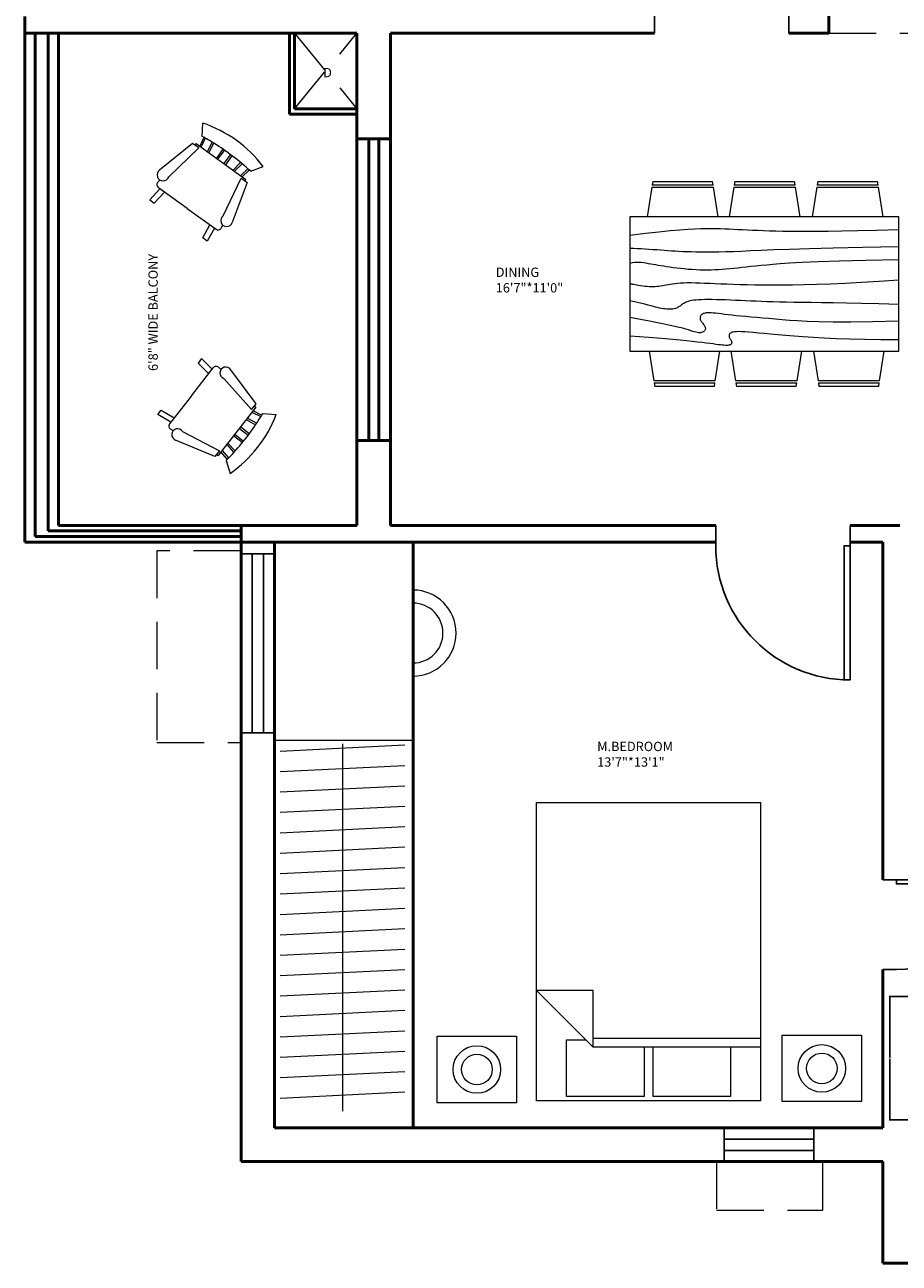
# Model space of a CAD drawing. Units: inches. Extents: x 4795 to 6024, y 2716 to 5025.
# Tile 9 of 19: x 4835 to 5069, y 3894 to 4226. Entities that reach past the tile are written whole.
import ezdxf

# ---------------------------------------------------------------- set-up
doc = ezdxf.new("R2010")
doc.units = ezdxf.units.IN
doc.linetypes.add('DASHED', pattern=[19.05, 12.7, -6.35])
for name, color, linetype, lineweight in [('A-ANNO-DIMS', 2, 'Continuous', 18), ('A-ANNO-TEXT', 7, 'Continuous', 18), ('A-AREA-IDEN', 3, 'Continuous', 18), ('A-DOOR', 4, 'Continuous', 25), ('A-FURN', 8, 'Continuous', 18), ('A-GLAZ', 4, 'Continuous', 25), ('A-WALL', 7, 'Continuous', 50), ('A-WALL-OVHD', 8, 'DASHED', 18)]:
    doc.layers.add(name, color=color, linetype=linetype, lineweight=lineweight)
doc.styles.get("Standard").update_dxf_attribs({"font": 'arial.ttf'})
doc.dimstyles.get("Standard").update_dxf_attribs({"dimtxt": 0.18, "dimasz": 0.18, "dimexe": 0.18, "dimexo": 0.0625, "dimgap": 0.09, "dimtad": 0, "dimtih": 1, "dimtoh": 1, "dimdec": 4, "dimzin": 0, "dimdsep": 46, "dimtxsty": 'Standard', "dimcen": 0.09, "dimadec": 0, "dimazin": 0, "dimtfac": 1, "dimtdec": 4, "dimtofl": 0, "dimtmove": 0, "dimatfit": 3, "dimfxl": 1, "dimtolj": 1, "dimtzin": 0, "dimarcsym": 0})

# ---------------------------------------------------------------- blocks, each defined once
blk = doc.blocks.new('*U2')
for p, q in [((0, 0), (0, -6)), ((40, 0), (40, -6))]:
    blk.add_line(p, q)
blk.add_lwpolyline([(0, 0), (0, 40), (1.75, 40), (1.75, 0)], close=True)
blk.add_arc((0, 0), 40, 0, 90)
blk = doc.blocks.new('Bed - Queen')
for p, q in [((0, -80.00003), (0, 0)), ((0, 0), (59.99999, 0)), ((59.99999, 0), (59.99999, -80.00003)), ((7.99999, -1.2), (28.79998, -1.2)), ((7.99999, -14.4), (7.99999, -1.2)), ((28.79998, -1.2), (28.79998, -14.4)), ((31.19999, -1.2), (51.99999, -1.2)), ((31.19999, -14.4), (31.19999, -1.2)), ((51.99999, -1.2), (51.99999, -16.4)), ((0, -14.4), (44.8, -14.4)), ((59.99999, -29.6), (44.8, -14.4)), ((44.8, -14.4), (44.8, -29.6)), ((51.99999, -16.4), (46.79936, -16.4)), ((44.8, -16.8), (0, -16.8)), ((44.8, -29.6), (59.99999, -29.6)), ((59.99999, -80.00003), (0, -80.00003))]:
    blk.add_line(p, q)
blk = doc.blocks.new('Chair - Rocking')
for p, q in [((-8, -4.5), (-10, -1.5)), ((8, -4.5), (10, -1.5)), ((-7.5, -4.5), (-7, -7)), ((-6.5, -7), (-7.02225, -4.43)), ((-4.5, -7), (-4.96674, -4.19951)), ((-4, -7), (-4.40532, -4.16272)), ((-1.5, -4.05012), (-1.5, -7)), ((-1, -7), (-1, -4.05012)), ((1, -7), (1, -4.04655)), ((1.5, -4.05012), (1.5, -7)), ((4, -7), (4.40187, -4.18694)), ((4.5, -7), (4.96761, -4.19437)), ((6.5, -7), (7, -4.4057)), ((7.5, -4.5), (7, -7)), ((-9, -7.5), (-12, -18.49999)), ((-7, -7.5), (-9, -7.5)), ((-9, -18.49999), (-7, -7.5)), ((-8.23428, -6.99939), (-8.3093, -7.47958)), ((-8.23041, -7), (8.23915, -7)), ((7, -7.5), (9, -7.5)), ((9, -18.49999), (7, -7.5)), ((8.31071, -7.48854), (8.23449, -7.00073)), ((9, -7.5), (12, -18.49999)), ((-10.36644, -20.64523), (-10.5, -21.49999)), ((-9, -22.49999), (-9.5, -26.49999)), ((0, -22.49999), (-9.5, -22.49999)), ((-8, -26.49999), (-7.5, -22.49999)), ((0, -22.49999), (9.5, -22.49999)), ((8, -26.49999), (7.5, -22.49999)), ((9, -22.49999), (9.5, -26.49999)), ((10.5, -21.49999), (10.3575, -20.58798)), ((-9.5, -26.49999), (-8, -26.49999)), ((9.5, -26.49999), (8, -26.49999))]:
    blk.add_line(p, q)
for centre, radius, start, end in [((0, -34.08333), 34.08333, 72.93847, 107.0615), ((0, -68.25004), 64.25, 93.92211, 97.15267), ((0, -68.25004), 64.25, 82.84733, 93.92211), ((-10.5, -18.99999), 1.58114, 161.5651, 18.43495), ((10.5, -18.99999), 1.58114, 161.5651, 18.43495), ((-9.5, -21.49999), 1, 180, 270), ((9.5, -21.49999), 1, 270, 0)]:
    blk.add_arc(centre, radius, start, end)
blk = doc.blocks.new('WIN-48')
for p, q in [((0, 0), (0, 48)), ((0, 48), (9, 48)), ((3, 0), (3, 48)), ((6, 48), (6, 0)), ((9, 48), (9, 0)), ((9, 0), (0, 0))]:
    blk.add_line(p, q)
blk = doc.blocks.new('WIN-24')
for p, q in [((0, 0), (0, 9)), ((0, 9), (24, 9)), ((24, 9), (24, 0)), ((0, 6), (24, 6)), ((24, 3), (0, 3)), ((24, 0), (0, 0))]:
    blk.add_line(p, q)
blk = doc.blocks.new('CHAIR-DINING')
for p, q in [((8, 17.72), (0, 18.97)), ((8, 17.71), (8, 1.25)), ((9.5, 17.48), (8.5, 17.64)), ((8.5, 1.33), (8.5, 17.64)), ((9.5, 17.48), (9.5, 1.48)), ((0, 0), (8, 1.25)), ((8.5, 1.33), (9.5, 1.48))]:
    blk.add_line(p, q)
blk = doc.blocks.new('*D27')
at = {"layer": 'A-ANNO-DIMS', "color": 0, "lineweight": -2, "transparency": 16777216}
for p, q in [((5071.7, 3965.06), (5066.63, 3965.06)), ((5066.81, 3964.88), (5066.81, 3948.72)), ((5066.81, 3932.19), (5066.81, 3948.35)), ((5071.7, 3932.01), (5066.63, 3932.01))]:
    blk.add_line(p, q, dxfattribs=at)
at = {"layer": 'A-ANNO-DIMS', "color": 0, "lineweight": 100, "transparency": 16777216}
for points in [[(5066.78, 3964.88), (5066.84, 3964.88), (5066.81, 3965.06)], [(5066.78, 3932.19), (5066.84, 3932.19), (5066.81, 3932.01)]]:
    blk.add_solid(points, dxfattribs=at)
at = {"layer": 'DEFPOINTS', "color": 0, "lineweight": 100, "transparency": 16777216}
for p in [(5071.76, 3965.06), (5066.81, 3932.01), (5071.76, 3932.01)]:
    blk.add_point(p, dxfattribs=at)
at = {"layer": 'A-ANNO-DIMS', "color": 0, "transparency": 16777216, "insert": (5066.81, 3948.53), "char_height": 0.18, "attachment_point": 5}
blk.add_mtext('\\A1;WC 33 TYP.', dxfattribs=at)

msp = doc.modelspace()

# ---------------------------------------------------------------- linework, layer by layer
at = {"layer": 'A-FURN'}
for p, q in [((5069.18, 4174.06), (4997.18, 4174.06)), ((4997.18, 4174.06), (4997.18, 4138.06)), ((5069.18, 4138.06), (5069.18, 4174.06)), ((4997.18, 4138.06), (5069.18, 4138.06)), ((4901.97, 4033.76), (4939.06, 4033.76)), ((4903.42, 4030.84), (4936.83, 4032.49)), ((4920.12, 4032.78), (4920.12, 3934.27)), ((4936.83, 4032.49), (4936.83, 4032.49)), ((4903.42, 4025.37), (4936.83, 4027.02)), ((4903.42, 4019.9), (4936.83, 4021.55)), ((4903.42, 4014.43), (4936.83, 4016.08)), ((4903.42, 4008.96), (4936.83, 4010.61)), ((4903.42, 4003.49), (4936.83, 4005.14)), ((4903.42, 3998.01), (4936.83, 3999.66)), ((4903.42, 3992.54), (4936.83, 3994.19)), ((4903.42, 3987.07), (4936.83, 3988.72)), ((4903.42, 3981.6), (4936.83, 3983.25)), ((4903.42, 3976.13), (4936.83, 3977.78)), ((4903.42, 3970.66), (4936.83, 3972.31)), ((4903.42, 3965.19), (4936.83, 3966.84)), ((4903.42, 3959.72), (4936.83, 3961.37)), ((4903.42, 3954.25), (4936.83, 3955.89)), ((4903.42, 3948.77), (4936.83, 3950.42)), ((4903.42, 3943.3), (4936.83, 3944.95)), ((4903.42, 3937.83), (4936.83, 3939.48))]:
    msp.add_line(p, q, dxfattribs=at)
for points in [[(5069.18, 4170.56), (5063.27, 4170.39), (5058.22, 4170.27), (5053.92, 4170.18), (5050.26, 4170.13), (5047.15, 4170.1), (5044.49, 4170.1), (5042.16, 4170.11), (5040.06, 4170.14), (5038.11, 4170.17), (5036.27, 4170.22), (5034.56, 4170.26), (5032.94, 4170.32), (5031.42, 4170.37), (5029.99, 4170.43), (5028.63, 4170.49), (5027.35, 4170.56), (5026.13, 4170.62), (5024.95, 4170.68), (5023.79, 4170.73), (5022.64, 4170.78), (5021.47, 4170.82), (5020.26, 4170.84), (5018.99, 4170.85), (5017.64, 4170.85), (5016.19, 4170.82), (5014.57, 4170.76), (5012.7, 4170.66), (5010.52, 4170.5), (5007.95, 4170.27), (5004.92, 4169.96), (5001.36, 4169.56), (4997.18, 4169.06)], [(5069.18, 4166.06), (5059.59, 4165.87), (5051.65, 4165.69), (5045.17, 4165.51), (5039.92, 4165.34), (5035.71, 4165.18), (5032.31, 4165.04), (5029.51, 4164.91), (5027.1, 4164.81), (5024.91, 4164.72), (5022.88, 4164.66), (5021.01, 4164.62), (5019.29, 4164.6), (5017.7, 4164.59), (5016.23, 4164.6), (5014.86, 4164.61), (5013.6, 4164.64), (5012.42, 4164.67), (5011.32, 4164.72), (5010.27, 4164.77), (5009.26, 4164.82), (5008.28, 4164.88), (5007.31, 4164.95), (5006.34, 4165.02), (5005.35, 4165.1), (5004.34, 4165.18), (5003.3, 4165.26), (5002.25, 4165.33), (5001.21, 4165.41), (5000.16, 4165.47), (4999.14, 4165.51), (4998.14, 4165.55), (4997.18, 4165.56)], [(5069.18, 4162.56), (5060.37, 4162.37), (5053.27, 4162.18), (5047.65, 4162), (5043.29, 4161.82), (5039.96, 4161.64), (5037.42, 4161.47), (5035.45, 4161.3), (5033.81, 4161.14), (5032.31, 4160.99), (5030.91, 4160.84), (5029.6, 4160.71), (5028.36, 4160.58), (5027.18, 4160.46), (5026.06, 4160.34), (5024.98, 4160.24), (5023.93, 4160.14), (5022.91, 4160.05), (5021.91, 4159.97), (5020.92, 4159.9), (5019.93, 4159.85), (5018.95, 4159.81), (5017.96, 4159.79), (5016.95, 4159.79), (5015.93, 4159.81), (5014.89, 4159.85), (5013.84, 4159.91), (5012.78, 4159.99), (5011.74, 4160.09), (5010.71, 4160.19), (5009.71, 4160.31), (5008.76, 4160.43), (5007.85, 4160.56), (5007.01, 4160.68), (5006.21, 4160.81), (5005.47, 4160.93), (5004.76, 4161.05), (5004.08, 4161.17), (5003.43, 4161.29), (5002.78, 4161.4), (5002.14, 4161.51), (5001.5, 4161.62), (5000.86, 4161.71), (5000.22, 4161.79), (4999.59, 4161.83), (4998.96, 4161.84), (4998.35, 4161.8), (4997.76, 4161.71), (4997.18, 4161.56)], [(5069.18, 4157.06), (5063.98, 4156.72), (5059.2, 4156.44), (5054.84, 4156.22), (5050.84, 4156.05), (5047.18, 4155.93), (5043.84, 4155.84), (5040.76, 4155.79), (5037.93, 4155.76), (5035.32, 4155.76), (5032.9, 4155.77), (5030.65, 4155.79), (5028.57, 4155.83), (5026.63, 4155.88), (5024.82, 4155.93), (5023.12, 4155.99), (5021.52, 4156.06), (5019.99, 4156.12), (5018.55, 4156.18), (5017.19, 4156.23), (5015.9, 4156.28), (5014.7, 4156.31), (5013.58, 4156.33), (5012.55, 4156.33), (5011.6, 4156.31), (5010.74, 4156.26), (5009.95, 4156.2), (5009.23, 4156.12), (5008.57, 4156.04), (5007.96, 4155.94), (5007.39, 4155.84), (5006.86, 4155.74), (5006.35, 4155.64), (5005.86, 4155.55), (5005.37, 4155.47), (5004.89, 4155.4), (5004.41, 4155.35), (5003.92, 4155.31), (5003.42, 4155.29), (5002.9, 4155.29), (5002.35, 4155.31), (5001.78, 4155.35), (5001.18, 4155.41), (5000.6, 4155.48), (5000.02, 4155.57), (4999.48, 4155.65), (4998.99, 4155.74), (4998.57, 4155.82), (4998.23, 4155.89), (4997.97, 4155.94), (4997.8, 4155.99), (4997.68, 4156.02), (4997.6, 4156.04), (4997.52, 4156.05), (4997.45, 4156.05), (4997.34, 4156.06), (4997.18, 4156.06)], [(5069.18, 4150.56), (5063.9, 4150.72), (5059.25, 4150.85), (5055.18, 4150.94), (5051.61, 4151), (5048.49, 4151.05), (5045.74, 4151.08), (5043.3, 4151.11), (5041.1, 4151.14), (5039.09, 4151.17), (5037.24, 4151.22), (5035.53, 4151.26), (5033.92, 4151.32), (5032.41, 4151.37), (5030.96, 4151.43), (5029.56, 4151.49), (5028.18, 4151.56), (5026.81, 4151.62), (5025.45, 4151.68), (5024.11, 4151.74), (5022.81, 4151.79), (5021.55, 4151.83), (5020.36, 4151.86), (5019.23, 4151.88), (5018.18, 4151.89), (5017.23, 4151.88), (5016.37, 4151.86), (5015.58, 4151.82), (5014.88, 4151.76), (5014.25, 4151.69), (5013.7, 4151.61), (5013.2, 4151.51), (5012.77, 4151.39), (5012.39, 4151.26), (5012.05, 4151.11), (5011.76, 4150.96), (5011.5, 4150.8), (5011.26, 4150.63), (5011.03, 4150.46), (5010.82, 4150.3), (5010.6, 4150.14), (5010.38, 4149.99), (5010.14, 4149.85), (5009.9, 4149.71), (5009.63, 4149.6), (5009.35, 4149.5), (5009.04, 4149.41), (5008.71, 4149.35), (5008.35, 4149.31), (5007.96, 4149.29), (5007.54, 4149.29), (5007.1, 4149.31), (5006.63, 4149.36), (5006.15, 4149.42), (5005.64, 4149.51), (5005.13, 4149.61), (5004.6, 4149.72), (5004.06, 4149.86), (5003.48, 4150.01), (5002.82, 4150.19), (5002.05, 4150.39), (5001.13, 4150.62), (5000.04, 4150.89), (4998.74, 4151.2), (4997.18, 4151.56)], [(5069.18, 4146.06), (5062.16, 4145.91), (5056.36, 4145.85), (5051.61, 4145.86), (5047.75, 4145.92), (5044.62, 4146.03), (5042.06, 4146.16), (5039.9, 4146.31), (5037.98, 4146.47), (5036.15, 4146.63), (5034.41, 4146.77), (5032.74, 4146.91), (5031.16, 4147.05), (5029.66, 4147.18), (5028.24, 4147.31), (5026.92, 4147.43), (5025.68, 4147.56), (5024.54, 4147.68), (5023.49, 4147.8), (5022.53, 4147.92), (5021.65, 4148.03), (5020.86, 4148.12), (5020.14, 4148.2), (5019.5, 4148.26), (5018.93, 4148.31), (5018.44, 4148.33), (5018, 4148.32), (5017.63, 4148.3), (5017.31, 4148.25), (5017.03, 4148.19), (5016.8, 4148.11), (5016.6, 4148.01), (5016.43, 4147.89), (5016.29, 4147.76), (5016.17, 4147.61), (5016.08, 4147.45), (5016.01, 4147.29), (5015.97, 4147.11), (5015.95, 4146.93), (5015.97, 4146.74), (5016.02, 4146.56), (5016.09, 4146.37), (5016.2, 4146.18), (5016.32, 4145.99), (5016.46, 4145.81), (5016.6, 4145.62), (5016.74, 4145.43), (5016.89, 4145.24), (5017.02, 4145.06), (5017.13, 4144.87), (5017.23, 4144.68), (5017.31, 4144.5), (5017.36, 4144.32), (5017.39, 4144.14), (5017.38, 4143.97), (5017.34, 4143.8), (5017.27, 4143.64), (5017.15, 4143.49), (5017.01, 4143.35), (5016.82, 4143.22), (5016.61, 4143.12), (5016.37, 4143.04), (5016.11, 4142.98), (5015.82, 4142.96), (5015.52, 4142.97), (5015.19, 4143.02), (5014.84, 4143.11), (5014.45, 4143.23), (5013.99, 4143.37), (5013.46, 4143.55), (5012.85, 4143.74), (5012.14, 4143.95), (5011.31, 4144.18), (5010.35, 4144.42), (5009.23, 4144.68), (5007.91, 4144.97), (5006.36, 4145.29), (5004.54, 4145.65), (5002.43, 4146.06), (4999.99, 4146.53), (4997.18, 4147.06)], [(5069.18, 4141.06), (5064.36, 4141.08), (5059.99, 4141.14), (5056.04, 4141.24), (5052.46, 4141.37), (5049.22, 4141.52), (5046.28, 4141.69), (5043.6, 4141.87), (5041.14, 4142.06), (5038.87, 4142.24), (5036.79, 4142.43), (5034.88, 4142.6), (5033.15, 4142.76), (5031.59, 4142.91), (5030.2, 4143.04), (5028.99, 4143.15), (5027.93, 4143.22), (5027.04, 4143.27), (5026.3, 4143.29), (5025.7, 4143.28), (5025.21, 4143.24), (5024.82, 4143.19), (5024.51, 4143.11), (5024.28, 4143.01), (5024.1, 4142.89), (5023.96, 4142.76), (5023.86, 4142.61), (5023.79, 4142.46), (5023.76, 4142.3), (5023.75, 4142.13), (5023.76, 4141.96), (5023.8, 4141.8), (5023.85, 4141.64), (5023.92, 4141.49), (5024, 4141.34), (5024.09, 4141.2), (5024.17, 4141.07), (5024.26, 4140.94), (5024.33, 4140.81), (5024.39, 4140.68), (5024.43, 4140.56), (5024.45, 4140.43), (5024.45, 4140.31), (5024.42, 4140.19), (5024.37, 4140.08), (5024.3, 4139.97), (5024.2, 4139.88), (5024.08, 4139.79), (5023.93, 4139.72), (5023.77, 4139.67), (5023.57, 4139.63), (5023.33, 4139.61), (5023.06, 4139.6), (5022.74, 4139.61), (5022.36, 4139.63), (5021.93, 4139.67), (5021.43, 4139.72), (5020.87, 4139.79), (5020.21, 4139.88), (5019.47, 4139.98), (5018.62, 4140.09), (5017.64, 4140.21), (5016.54, 4140.34), (5015.29, 4140.49), (5013.89, 4140.64), (5012.33, 4140.8), (5010.6, 4140.97), (5008.71, 4141.14), (5006.68, 4141.32), (5004.5, 4141.5), (5002.19, 4141.68), (4999.75, 4141.87), (4997.18, 4142.06)]]:
    msp.add_lwpolyline(points, dxfattribs=at)
for points in [[(4945.53, 3954.4), (4966.79, 3954.4), (4966.79, 3936.56), (4945.53, 3936.56)], [(5037.96, 3954.7), (5059.23, 3954.7), (5059.23, 3936.87), (5037.96, 3936.87)]]:
    msp.add_lwpolyline(points, close=True, dxfattribs=at)
for centre, radius in [((4956.16, 3945.48), 6.37), ((5048.6, 3945.78), 6.37), ((4956.16, 3945.48), 4.11), ((5048.6, 3945.78), 4.11)]:
    msp.add_circle(centre, radius, dxfattribs=at)
for radius in [11.53, 8.02]:
    msp.add_arc((4939.06, 4062.48), radius, 270, 90, dxfattribs=at)
at = {"layer": 'A-WALL'}
for p, q in [((5050.47, 4271.31), (5050.47, 4223.31)), ((4835.02, 4227.81), (4835.02, 4223.31)), ((4835.02, 4223.31), (4835.02, 4086.81)), ((4892.97, 4223.31), (4835.02, 4223.31)), ((4837.81, 4223.31), (4837.81, 4088.33)), ((4841.3, 4223.31), (4841.3, 4089.92)), ((4844.02, 4223.31), (4844.02, 4091.31)), ((4924.02, 4223.31), (4892.97, 4223.31)), ((4905.94, 4223.31), (4905.94, 4201.63)), ((4907.27, 4223.31), (4907.27, 4203.01)), ((4924.02, 4223.31), (4924.02, 4091.31)), ((4933.02, 4223.31), (4933.02, 4091.31)), ((5003.74, 4223.31), (4933.02, 4223.31)), ((5050.47, 4223.31), (5039.74, 4223.31)), ((4905.94, 4201.63), (4924.02, 4201.63)), ((4907.27, 4203.01), (4924.02, 4203.01)), ((4924.02, 4194.96), (4933.02, 4194.96)), ((4927.18, 4194.96), (4927.18, 4114.12)), ((4929.9, 4194.96), (4929.9, 4114.12)), ((4924.02, 4114.12), (4933.02, 4114.12)), ((4892.97, 4091.31), (4844.02, 4091.31)), ((4892.97, 4091.31), (4892.97, 3920.81)), ((4924.02, 4091.31), (4892.97, 4091.31)), ((5020.15, 4091.31), (4933.02, 4091.31)), ((5069.47, 4091.31), (5056.15, 4091.31)), ((4837.81, 4088.33), (4892.97, 4088.33)), ((4841.3, 4089.92), (4892.97, 4089.92)), ((4892.97, 4086.81), (4835.02, 4086.81)), ((5020.15, 4086.81), (4892.97, 4086.81)), ((4901.97, 4086.81), (4901.97, 3929.81)), ((4939.06, 4086.81), (4939.06, 3929.81)), ((5064.97, 4086.81), (5056.15, 4086.81)), ((5064.97, 4086.81), (5064.97, 3996.29)), ((5064.97, 3972.29), (5064.97, 3929.81)), ((5064.97, 3929.81), (4901.97, 3929.81)), ((5064.97, 3920.81), (4892.97, 3920.81)), ((5064.97, 3920.81), (5064.97, 3893.55)), ((5064.97, 3893.55), (5152.97, 3893.55))]:
    msp.add_line(p, q, dxfattribs=at)
at = {"layer": 'A-WALL-OVHD'}
for p, q in [((4907.27, 4223.31), (4924.02, 4203.01)), ((4907.27, 4203.01), (4924.02, 4223.31)), ((5050.47, 4223.31), (5129.47, 4223.31)), ((4892.97, 4084.57), (4870.38, 4084.57)), ((4870.38, 4084.57), (4870.38, 4033.16)), ((4870.38, 4033.16), (4892.97, 4033.16)), ((5020.38, 3920.81), (5020.38, 3907.81)), ((5048.87, 3907.81), (5048.87, 3920.81)), ((5020.38, 3907.81), (5048.87, 3907.81))]:
    msp.add_line(p, q, dxfattribs=at)

# ---------------------------------------------------------------- block references
at = {"layer": 'A-DOOR', "xscale": -0.9, "yscale": 0.9, "zscale": 0.9}
msp.add_blockref('*U2', (5039.74, 4228.71), dxfattribs=at)
at = {"layer": 'A-DOOR'}
for p, xscale, yscale, zscale, rotation in [((5056.15, 4085.91), 0.9, 0.9, 0.9, 180), ((5068.57, 3996.29), 0.6, 0.6, 0.6, 270)]:
    msp.add_blockref('*U2', p, dxfattribs=dict(at, xscale=xscale, yscale=yscale, zscale=zscale, rotation=rotation))
at = {"layer": 'A-FURN'}
for name, p, rotation in [('Chair - Rocking', (4891.68, 4194.59), 324.2775344515209), ('CHAIR-DINING', (5020.79, 4174.06), 90.00567182442555), ('CHAIR-DINING', (5042.76, 4174.06), 90.00567182442285), ('CHAIR-DINING', (5064.99, 4174.06), 90.0056718244202), ('Chair - Rocking', (4897.41, 4112.25), 232.0049313276433), ('CHAIR-DINING', (5002.32, 4138.06), 270.0000000000027), ('CHAIR-DINING', (5024.25, 4138.06), 270), ('CHAIR-DINING', (5046.35, 4138.06), 269.9999999999973), ('Bed - Queen', (5032.16, 3937.06), 180)]:
    msp.add_blockref(name, p, dxfattribs=dict(at, rotation=rotation))
at = {"layer": 'A-GLAZ', "rotation": 180}
for name, p in [('WIN-48', (4901.98, 4083.74)), ('WIN-24', (5046.45, 3929.81))]:
    msp.add_blockref(name, p, dxfattribs=at)

# ---------------------------------------------------------------- texts
at = {"layer": 'A-ANNO-TEXT', "insert": (4914.96, 4213.98), "char_height": 2.5, "attachment_point": 1}
msp.add_mtext_dynamic_manual_height_columns('D', width=1.8574, gutter_width=12.5, heights=[0], dxfattribs=at)
at = {"layer": 'A-AREA-IDEN', "insert": (4868.15, 4132.75), "char_height": 2.5, "attachment_point": 1, "rotation": 90}
msp.add_mtext_dynamic_manual_height_columns('6\'8" WIDE BALCONY', width=54.8875, gutter_width=12.5, heights=[0], dxfattribs=at)
at = {"layer": 'A-AREA-IDEN', "char_height": 2.5, "attachment_point": 1}
for s, width, insert in [('DINING\\P16\'7"*11\'0"', 42.6658, (4961.22, 4160.46)), ('M.BEDROOM\\P13\'7"*13\'1"', 69.0887, (4988.4, 4033.34))]:
    msp.add_mtext_dynamic_manual_height_columns(s, width=width, gutter_width=12.5, heights=[0], dxfattribs=dict(at, insert=insert))

# ---------------------------------------------------------------- dimensions: what is measured, and where the dimension line sits
at = {"layer": 'A-ANNO-DIMS'}
dim = msp.add_linear_dim(base=(5066.81, 3932.01), p1=(5071.76, 3965.06), p2=(5071.76, 3932.01), angle=270, text='WC <> TYP.', dimstyle='Standard', override={"dimdec": 0, "dimlfac": 1, "dimrnd": 0, "dimzin": 0, "dimdsep": 46, "dimlunit": 2}, dxfattribs=at)
dim.commit()
dim.dimension.update_dxf_attribs({"geometry": '*D27', "text_midpoint": (5066.81, 3948.53)})

doc.saveas('drawing.dxf')
